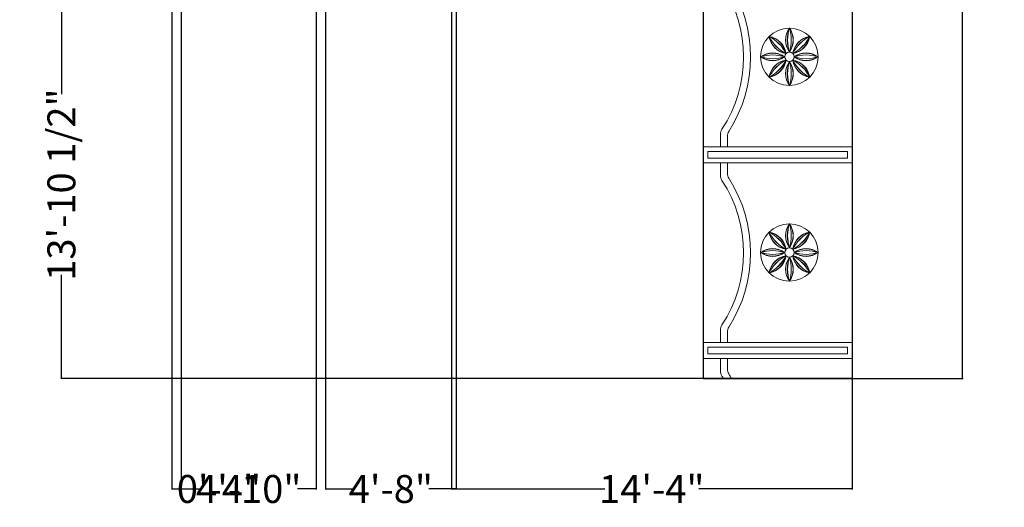
# Model space of a CAD drawing. Units: inches. Extents: x 1146 to 2917, y 889 to 2437.
# Tile 10 of 13: x 2395 to 2817, y 1377 to 1586. Entities that reach past the tile are written whole.
import ezdxf

# ---------------------------------------------------------------- set-up
doc = ezdxf.new("R2010")
doc.units = ezdxf.units.IN
doc.header["$MEASUREMENT"] = 0
for name, color, linetype, lineweight in [('A-ANNO-DIMS', 2, 'Continuous', 18), ('A-ELEV', 7, 'Continuous', 30), ('A-ELEV-ORNM', 8, 'Continuous', 18)]:
    doc.layers.add(name, color=color, linetype=linetype, lineweight=lineweight)
doc.styles.get("Standard").update_dxf_attribs({"font": 'arial.ttf'})
doc.dimstyles.get("Standard").update_dxf_attribs({"dimtxt": 12, "dimasz": 0.18, "dimexe": 0.18, "dimexo": 0.0625, "dimgap": 0.09, "dimtad": 0, "dimtoh": 1, "dimdec": 1, "dimzin": 0, "dimdsep": 46, "dimlunit": 4, "dimtxsty": 'Standard', "dimcen": 0.09, "dimadec": 0, "dimazin": 0, "dimtfac": 1, "dimtdec": 1, "dimtofl": 0, "dimtmove": 0, "dimatfit": 3, "dimfxl": 1, "dimtolj": 1, "dimtzin": 0, "dimarcsym": 0})

# ---------------------------------------------------------------- blocks, each defined once
blk = doc.blocks.new('BOUNDARY-WALL-PIER')
for points in [[(0, 6.94), (64, 6.94), (64, 0), (0, 0)], [(2, 4.94), (62, 4.94), (62, 2), (2, 2)]]:
    blk.add_lwpolyline(points, close=True)
blk = doc.blocks.new('BOUNDARY-WALL-ARCH-CAP')
for p, q in [((0, 71.74), (0, 77.06)), ((3, 72.62), (3, 77.06)), ((0, 0), (0, 5.32)), ((3, 0), (3, 4.44))]:
    blk.add_line(p, q)
for centre, radius, start, end in [((7, 72.62), 4, 180, 212.2708), ((4, 71.74), 4, 180, 213.079), ((-46.98, 38.53), 56.85, 326.921, 33.079), ((-46.98, 38.53), 59.85, 327.7292, 32.2708), ((4, 5.32), 4, 146.921, 180), ((7, 4.44), 4, 147.7292, 180)]:
    blk.add_arc(centre, radius, start, end)
blk = doc.blocks.new('ROSETTE-PLANAR-TRACERY')
for radius in [12.33, 2.02]:
    blk.add_circle((12.33, 12.33), radius)
at = {"extrusion": (-2e-16, 0, -1)}
for centre, radius, start, end in [((-19.47, 19.51), 8.8, 324.1552, 35.8448), ((-4.71, 19.51), 9.21, 145.95, 214.05)]:
    blk.add_arc(centre, radius, start, end, dxfattribs=at)
for centre, radius, start, end in [((19.96, 19.51), 9.21, 145.95, 214.05), ((5.2, 19.51), 8.8, 324.1552, 35.8448), ((2.21, 12.37), 8.8, 9.1552, 80.8448), ((12.65, 22.8), 9.21, 190.95, 259.05), ((12.37, 22.46), 8.8, 279.1552, 350.8448), ((22.8, 12.02), 9.21, 100.95, 169.05), ((5.15, 5.2), 8.8, 54.1552, 125.8448), ((19.51, 4.71), 9.21, 55.95, 124.05), ((5.15, 19.96), 9.21, 235.95, 304.05), ((12.3, 2.21), 8.8, 99.1552, 170.8448), ((1.86, 12.65), 9.21, 280.95, 349.05), ((19.47, 5.15), 8.8, 144.1552, 215.8448), ((4.71, 5.15), 9.21, 325.95, 34.05), ((22.46, 12.3), 8.8, 189.1552, 260.8448), ((12.02, 1.86), 9.21, 10.95, 79.05), ((19.51, 19.47), 8.8, 234.1552, 305.8448)]:
    blk.add_arc(centre, radius, start, end)
at = {"extrusion": (-2e-16, -2e-16, -1)}
for centre, radius, start, end in [((-12.3, 22.46), 8.8, 279.1552, 350.8448), ((-1.86, 12.02), 9.21, 100.95, 169.05)]:
    blk.add_arc(centre, radius, start, end, dxfattribs=at)
at = {"extrusion": (-2e-16, 2e-16, -1)}
for centre, radius, start, end in [((-22.46, 12.37), 8.8, 9.1552, 80.8448), ((-12.02, 22.8), 9.21, 190.95, 259.05)]:
    blk.add_arc(centre, radius, start, end, dxfattribs=at)
at = {"extrusion": (0, -2e-16, -1)}
for centre, radius, start, end in [((-5.15, 4.71), 9.21, 55.95, 124.05), ((-5.15, 19.47), 8.8, 234.1552, 305.8448)]:
    blk.add_arc(centre, radius, start, end, dxfattribs=at)
at = {"extrusion": (0, 2e-16, -1)}
for centre, radius, start, end in [((-19.51, 5.2), 8.8, 54.1552, 125.8448), ((-19.51, 19.96), 9.21, 235.95, 304.05)]:
    blk.add_arc(centre, radius, start, end, dxfattribs=at)
at = {"extrusion": (2e-16, -2e-16, -1)}
for centre, radius, start, end in [((-2.21, 12.3), 8.8, 189.1552, 260.8448), ((-12.65, 1.86), 9.21, 10.95, 79.05)]:
    blk.add_arc(centre, radius, start, end, dxfattribs=at)
at = {"extrusion": (2e-16, 0, -1)}
for centre, radius, start, end in [((-19.96, 5.15), 9.21, 325.95, 34.05), ((-5.2, 5.15), 8.8, 144.1552, 215.8448)]:
    blk.add_arc(centre, radius, start, end, dxfattribs=at)
at = {"extrusion": (2e-16, 2e-16, -1)}
for centre, radius, start, end in [((-12.37, 2.21), 8.8, 99.1552, 170.8448), ((-22.8, 12.65), 9.21, 280.95, 349.05)]:
    blk.add_arc(centre, radius, start, end, dxfattribs=at)
blk = doc.blocks.new('*D121')
at = {"layer": 'A-ANNO-DIMS', "color": 0, "lineweight": -2, "transparency": 16777216}
for p, q in [((2752.26, 2371.39), (2799.78, 2371.39)), ((2799.6, 2371.21), (2799.6, 1936.27)), ((2799.6, 1432.07), (2799.6, 1867.01)), ((2752.26, 1431.89), (2799.78, 1431.89))]:
    blk.add_line(p, q, dxfattribs=at)
at = {"layer": 'A-ANNO-DIMS', "color": 0, "transparency": 16777216}
for points in [[(2799.57, 2371.21), (2799.63, 2371.21), (2799.6, 2371.39)], [(2799.57, 1432.07), (2799.63, 1432.07), (2799.6, 1431.89)]]:
    blk.add_solid(points, dxfattribs=at)
at = {"layer": 'Defpoints', "color": 0, "transparency": 16777216}
for p in [(2752.2, 2371.39), (2799.6, 2371.39), (2752.2, 1431.89)]:
    blk.add_point(p, dxfattribs=at)
at = {"layer": 'A-ANNO-DIMS', "color": 0, "transparency": 16777216, "insert": (2799.6, 1901.64), "char_height": 12, "attachment_point": 5, "rotation": 90}
blk.add_mtext('\\A1;78\'-3 1/2"', dxfattribs=at)
blk = doc.blocks.new('*D128')
at = {"layer": 'A-ANNO-DIMS', "color": 0, "lineweight": -2, "transparency": 16777216}
for p, q in [((2580.2, 1598.33), (2580.2, 1384.31)), ((2752.2, 1431.83), (2752.2, 1384.31)), ((2580.38, 1384.49), (2646.06, 1384.49)), ((2752.02, 1384.49), (2686.34, 1384.49))]:
    blk.add_line(p, q, dxfattribs=at)
at = {"layer": 'A-ANNO-DIMS', "color": 0, "transparency": 16777216}
for points in [[(2580.38, 1384.52), (2580.38, 1384.46), (2580.2, 1384.49)], [(2752.02, 1384.52), (2752.02, 1384.46), (2752.2, 1384.49)]]:
    blk.add_solid(points, dxfattribs=at)
at = {"layer": 'Defpoints', "color": 0, "transparency": 16777216}
for p in [(2580.2, 1598.39), (2752.2, 1431.89), (2752.2, 1384.49)]:
    blk.add_point(p, dxfattribs=at)
at = {"layer": 'A-ANNO-DIMS', "color": 0, "transparency": 16777216, "insert": (2666.2, 1384.49), "char_height": 12, "attachment_point": 5}
blk.add_mtext('\\A1;14\'-4"', dxfattribs=at)
blk = doc.blocks.new('*D129')
at = {"layer": 'A-ANNO-DIMS', "color": 0, "lineweight": -2, "transparency": 16777216}
for p, q in [((2580.14, 1598.39), (2412.62, 1598.39)), ((2412.8, 1598.21), (2412.8, 1553.92)), ((2412.8, 1432.07), (2412.8, 1476.36)), ((2752.14, 1431.89), (2412.62, 1431.89))]:
    blk.add_line(p, q, dxfattribs=at)
at = {"layer": 'A-ANNO-DIMS', "color": 0, "transparency": 16777216}
for points in [[(2412.77, 1598.21), (2412.83, 1598.21), (2412.8, 1598.39)], [(2412.77, 1432.07), (2412.83, 1432.07), (2412.8, 1431.89)]]:
    blk.add_solid(points, dxfattribs=at)
at = {"layer": 'Defpoints', "color": 0, "transparency": 16777216}
for p in [(2580.2, 1598.39), (2412.8, 1431.89), (2752.2, 1431.89)]:
    blk.add_point(p, dxfattribs=at)
at = {"layer": 'A-ANNO-DIMS', "color": 0, "transparency": 16777216, "insert": (2412.8, 1515.14), "char_height": 12, "attachment_point": 5, "rotation": 90}
blk.add_mtext('\\A1;13\'-10 1/2"', dxfattribs=at)
blk = doc.blocks.new('*D133')
at = {"layer": 'A-ANNO-DIMS', "color": 0, "lineweight": -2, "transparency": 16777216}
for p, q in [((2464.2, 1865.33), (2464.2, 1384.31)), ((2522.2, 1865.33), (2522.2, 1384.31)), ((2464.38, 1384.49), (2472.26, 1384.49)), ((2522.02, 1384.49), (2514.14, 1384.49))]:
    blk.add_line(p, q, dxfattribs=at)
at = {"layer": 'A-ANNO-DIMS', "color": 0, "transparency": 16777216}
for points in [[(2464.38, 1384.52), (2464.38, 1384.46), (2464.2, 1384.49)], [(2522.02, 1384.52), (2522.02, 1384.46), (2522.2, 1384.49)]]:
    blk.add_solid(points, dxfattribs=at)
at = {"layer": 'Defpoints', "color": 0, "transparency": 16777216}
for p in [(2464.2, 1865.39), (2522.2, 1865.39), (2522.2, 1384.49)]:
    blk.add_point(p, dxfattribs=at)
at = {"layer": 'A-ANNO-DIMS', "color": 0, "transparency": 16777216, "insert": (2493.2, 1384.49), "char_height": 12, "attachment_point": 5}
blk.add_mtext('\\A1;4\'-10"', dxfattribs=at)
blk = doc.blocks.new('*D134')
at = {"layer": 'A-ANNO-DIMS', "color": 0, "lineweight": -2, "transparency": 16777216}
for p, q in [((2526.2, 1865.33), (2526.2, 1384.31)), ((2582.2, 1865.33), (2582.2, 1384.31)), ((2526.38, 1384.49), (2537.92, 1384.49)), ((2582.02, 1384.49), (2570.48, 1384.49))]:
    blk.add_line(p, q, dxfattribs=at)
at = {"layer": 'A-ANNO-DIMS', "color": 0, "transparency": 16777216}
for points in [[(2526.38, 1384.52), (2526.38, 1384.46), (2526.2, 1384.49)], [(2582.02, 1384.52), (2582.02, 1384.46), (2582.2, 1384.49)]]:
    blk.add_solid(points, dxfattribs=at)
at = {"layer": 'Defpoints', "color": 0, "transparency": 16777216}
for p in [(2526.2, 1865.39), (2582.2, 1865.39), (2582.2, 1384.49)]:
    blk.add_point(p, dxfattribs=at)
at = {"layer": 'A-ANNO-DIMS', "color": 0, "transparency": 16777216, "insert": (2554.2, 1384.49), "char_height": 12, "attachment_point": 5}
blk.add_mtext('\\A1;4\'-8"', dxfattribs=at)
blk = doc.blocks.new('*D135')
at = {"layer": 'A-ANNO-DIMS', "color": 0, "lineweight": -2, "transparency": 16777216}
for p, q in [((2460.2, 1869.33), (2460.2, 1384.31)), ((2464.2, 1865.33), (2464.2, 1384.31)), ((2460.38, 1384.49), (2464.02, 1384.49)), ((2464.2, 1384.49), (2464.38, 1384.49))]:
    blk.add_line(p, q, dxfattribs=at)
at = {"layer": 'A-ANNO-DIMS', "color": 0, "transparency": 16777216}
for points in [[(2460.38, 1384.52), (2460.38, 1384.46), (2460.2, 1384.49)], [(2464.02, 1384.52), (2464.02, 1384.46), (2464.2, 1384.49)]]:
    blk.add_solid(points, dxfattribs=at)
at = {"layer": 'Defpoints', "color": 0, "transparency": 16777216}
for p in [(2460.2, 1869.39), (2464.2, 1865.39), (2464.2, 1384.49)]:
    blk.add_point(p, dxfattribs=at)
at = {"layer": 'A-ANNO-DIMS', "color": 0, "transparency": 16777216, "insert": (2480.42, 1384.49), "char_height": 12, "attachment_point": 5}
blk.add_mtext('\\A1;0\'-4"', dxfattribs=at)

msp = doc.modelspace()

# ---------------------------------------------------------------- linework, layer by layer
at = {"layer": 'A-ELEV'}
for p, q in [((2752.2, 2371.39), (2752.2, 1431.89)), ((2688.2, 2182.39), (2688.2, 1431.89)), ((2688.2, 1431.89), (2752.2, 1431.89))]:
    msp.add_line(p, q, dxfattribs=at)
at = {"layer": 'A-ELEV-ORNM'}
for p, q in [((2695.67, 1435.13), (2695.67, 1440.45)), ((2698.67, 1436.01), (2698.67, 1440.45))]:
    msp.add_line(p, q, dxfattribs=at)
at = {"layer": 'A-ELEV-ORNM', "extrusion": (0.866025, 5.48447e-11, -0.5)}
for centre, radius, start, end in [((1577.18, 1369.76, 2360.14), 8.8, 234.1552, 305.8448), ((1577.18, 1355, 2360.14), 9.21, 55.95, 124.05), ((1493.18, 1369.76, 2360.14), 8.8, 234.1552, 305.8448), ((1493.18, 1355, 2360.14), 9.21, 55.95, 124.05)]:
    msp.add_arc(centre, radius, start, end, dxfattribs=at)
at = {"layer": 'A-ELEV-ORNM', "extrusion": (-0.866025, -5.48447e-11, -0.5)}
for centre, radius, start, end in [((-1577.18, -1369.76, -2360.14), 8.8, 54.1552, 125.8448), ((-1577.18, -1355, -2360.14), 9.21, 235.95, 304.05), ((-1493.18, -1369.76, -2360.14), 8.8, 54.1552, 125.8448), ((-1493.18, -1355, -2360.14), 9.21, 235.95, 304.05)]:
    msp.add_arc(centre, radius, start, end, dxfattribs=at)
at = {"layer": 'A-ELEV-ORNM', "extrusion": (0.866025, 5.48447e-11, 0.5)}
for centre, radius, start, end in [((1577.18, -1370.26, 2360.14), 9.21, 55.95, 124.05), ((1577.18, -1355.49, 2360.14), 8.8, 234.1552, 305.8448), ((1493.18, -1370.26, 2360.14), 9.21, 55.95, 124.05), ((1493.18, -1355.49, 2360.14), 8.8, 234.1552, 305.8448)]:
    msp.add_arc(centre, radius, start, end, dxfattribs=at)
at = {"layer": 'A-ELEV-ORNM', "extrusion": (-0.866025, -5.48447e-11, 0.5)}
for centre, radius, start, end in [((-1577.18, 1370.26, -2360.14), 9.21, 235.95, 304.05), ((-1577.18, 1355.49, -2360.14), 8.8, 54.1552, 125.8448), ((-1493.18, 1370.26, -2360.14), 9.21, 235.95, 304.05), ((-1493.18, 1355.49, -2360.14), 8.8, 54.1552, 125.8448)]:
    msp.add_arc(centre, radius, start, end, dxfattribs=at)
at = {"layer": 'A-ELEV-ORNM', "extrusion": (0.612372, 0.612372, 0.5)}
for centre, radius, start, end in [((-809.71, -1511.47, 2630.3), 8.8, 234.1552, 305.8448), ((-809.71, -1526.23, 2630.3), 9.21, 55.95, 124.05), ((-824.07, -1525.74, 2630.3), 8.8, 54.1552, 125.8448), ((-824.07, -1510.98, 2630.3), 9.21, 235.95, 304.05), ((-869.1, -1481.77, 2578.86), 8.8, 234.1552, 305.8448), ((-869.1, -1496.53, 2578.86), 9.21, 55.95, 124.05), ((-883.46, -1496.04, 2578.86), 8.8, 54.1552, 125.8448), ((-883.46, -1481.28, 2578.86), 9.21, 235.95, 304.05)]:
    msp.add_arc(centre, radius, start, end, dxfattribs=at)
at = {"layer": 'A-ELEV-ORNM', "extrusion": (0.612372, 0.612372, -0.5)}
for centre, radius, start, end in [((-809.71, 1525.74, 2630.3), 8.8, 234.1552, 305.8448), ((-809.71, 1510.98, 2630.3), 9.21, 55.95, 124.05), ((-824.07, 1511.47, 2630.3), 8.8, 54.1552, 125.8448), ((-824.07, 1526.23, 2630.3), 9.21, 235.95, 304.05), ((-869.1, 1496.04, 2578.86), 8.8, 234.1552, 305.8448), ((-869.1, 1481.28, 2578.86), 9.21, 55.95, 124.05), ((-883.46, 1481.77, 2578.86), 8.8, 54.1552, 125.8448), ((-883.46, 1496.53, 2578.86), 9.21, 235.95, 304.05)]:
    msp.add_arc(centre, radius, start, end, dxfattribs=at)
at = {"layer": 'A-ELEV-ORNM', "extrusion": (-0.612372, -0.612372, -0.5)}
for centre, radius, start, end in [((809.71, -1525.74, -2630.3), 8.8, 54.1552, 125.8448), ((809.71, -1510.98, -2630.3), 9.21, 235.95, 304.05), ((824.07, -1511.47, -2630.3), 8.8, 234.1552, 305.8448), ((824.07, -1526.23, -2630.3), 9.21, 55.95, 124.05), ((869.1, -1496.04, -2578.86), 8.8, 54.1552, 125.8448), ((869.1, -1481.28, -2578.86), 9.21, 235.95, 304.05), ((883.46, -1481.77, -2578.86), 8.8, 234.1552, 305.8448), ((883.46, -1496.53, -2578.86), 9.21, 55.95, 124.05)]:
    msp.add_arc(centre, radius, start, end, dxfattribs=at)
at = {"layer": 'A-ELEV-ORNM', "extrusion": (-0.612372, -0.612372, 0.5)}
for centre, radius, start, end in [((809.71, 1511.47, -2630.3), 8.8, 54.1552, 125.8448), ((809.71, 1526.23, -2630.3), 9.21, 235.95, 304.05), ((824.07, 1525.74, -2630.3), 8.8, 234.1552, 305.8448), ((824.07, 1510.98, -2630.3), 9.21, 55.95, 124.05), ((869.1, 1481.77, -2578.86), 8.8, 54.1552, 125.8448), ((869.1, 1496.53, -2578.86), 9.21, 235.95, 304.05), ((883.46, 1496.04, -2578.86), 8.8, 234.1552, 305.8448), ((883.46, 1481.28, -2578.86), 9.21, 55.95, 124.05)]:
    msp.add_arc(centre, radius, start, end, dxfattribs=at)
at = {"layer": 'A-ELEV-ORNM', "extrusion": (0.612372, -0.612372, 0.5)}
for centre, radius, start, end in [((3044.39, -401.31, 707.45), 8.8, 234.1552, 305.8448), ((3044.39, -416.07, 707.45), 9.21, 55.95, 124.05), ((3030.03, -415.58, 707.45), 8.8, 54.1552, 125.8448), ((3030.03, -400.82, 707.45), 9.21, 235.95, 304.05), ((2984.99, -431.01, 758.88), 8.8, 234.1552, 305.8448), ((2984.99, -445.77, 758.88), 9.21, 55.95, 124.05), ((2970.63, -445.28, 758.88), 8.8, 54.1552, 125.8448), ((2970.63, -430.51, 758.88), 9.21, 235.95, 304.05)]:
    msp.add_arc(centre, radius, start, end, dxfattribs=at)
at = {"layer": 'A-ELEV-ORNM', "extrusion": (0.612372, -0.612372, -0.5)}
for centre, radius, start, end in [((3044.39, 415.58, 707.45), 8.8, 234.1552, 305.8448), ((3044.39, 400.82, 707.45), 9.21, 55.95, 124.05), ((3030.03, 401.31, 707.45), 8.8, 54.1552, 125.8448), ((3030.03, 416.07, 707.45), 9.21, 235.95, 304.05), ((2984.99, 445.28, 758.88), 8.8, 234.1552, 305.8448), ((2984.99, 430.51, 758.88), 9.21, 55.95, 124.05), ((2970.63, 431.01, 758.88), 8.8, 54.1552, 125.8448), ((2970.63, 445.77, 758.88), 9.21, 235.95, 304.05)]:
    msp.add_arc(centre, radius, start, end, dxfattribs=at)
at = {"layer": 'A-ELEV-ORNM', "extrusion": (-0.612372, 0.612372, -0.5)}
for centre, radius, start, end in [((-3044.39, -415.58, -707.45), 8.8, 54.1552, 125.8448), ((-3044.39, -400.82, -707.45), 9.21, 235.95, 304.05), ((-3030.03, -401.31, -707.45), 8.8, 234.1552, 305.8448), ((-3030.03, -416.07, -707.45), 9.21, 55.95, 124.05), ((-2984.99, -445.28, -758.88), 8.8, 54.1552, 125.8448), ((-2984.99, -430.51, -758.88), 9.21, 235.95, 304.05), ((-2970.63, -431.01, -758.88), 8.8, 234.1552, 305.8448), ((-2970.63, -445.77, -758.88), 9.21, 55.95, 124.05)]:
    msp.add_arc(centre, radius, start, end, dxfattribs=at)
at = {"layer": 'A-ELEV-ORNM', "extrusion": (-0.612372, 0.612372, 0.5)}
for centre, radius, start, end in [((-3044.39, 401.31, -707.45), 8.8, 54.1552, 125.8448), ((-3044.39, 416.07, -707.45), 9.21, 235.95, 304.05), ((-3030.03, 415.58, -707.45), 8.8, 234.1552, 305.8448), ((-3030.03, 400.82, -707.45), 9.21, 55.95, 124.05), ((-2984.99, 431.01, -758.88), 8.8, 54.1552, 125.8448), ((-2984.99, 445.77, -758.88), 9.21, 235.95, 304.05), ((-2970.63, 445.28, -758.88), 8.8, 234.1552, 305.8448), ((-2970.63, 430.51, -758.88), 9.21, 55.95, 124.05)]:
    msp.add_arc(centre, radius, start, end, dxfattribs=at)
at = {"layer": 'A-ELEV-ORNM', "extrusion": (-5.48444e-11, 0.866025, 0.5)}
for centre, radius, start, end in [((-2718.08, -777.87, 1359.66), 8.8, 234.1552, 305.8448), ((-2718.08, -792.63, 1359.66), 9.21, 55.95, 124.05), ((-2732.44, -777.37, 1359.66), 9.21, 235.95, 304.05), ((-2732.44, -792.14, 1359.66), 8.8, 54.1552, 125.8448), ((-2718.08, -735.87, 1286.92), 8.8, 234.1552, 305.8448), ((-2718.08, -750.63, 1286.92), 9.21, 55.95, 124.05), ((-2732.44, -735.37, 1286.92), 9.21, 235.95, 304.05), ((-2732.44, -750.14, 1286.92), 8.8, 54.1552, 125.8448)]:
    msp.add_arc(centre, radius, start, end, dxfattribs=at)
at = {"layer": 'A-ELEV-ORNM', "extrusion": (5.48444e-11, -0.866025, 0.5)}
for centre, radius, start, end in [((2718.08, 777.87, -1359.66), 8.8, 54.1552, 125.8448), ((2718.08, 792.63, -1359.66), 9.21, 235.95, 304.05), ((2732.44, 777.37, -1359.66), 9.21, 55.95, 124.05), ((2732.44, 792.14, -1359.66), 8.8, 234.1552, 305.8448), ((2718.08, 735.87, -1286.92), 8.8, 54.1552, 125.8448), ((2718.08, 750.63, -1286.92), 9.21, 235.95, 304.05), ((2732.44, 735.37, -1286.92), 9.21, 55.95, 124.05), ((2732.44, 750.14, -1286.92), 8.8, 234.1552, 305.8448)]:
    msp.add_arc(centre, radius, start, end, dxfattribs=at)
at = {"layer": 'A-ELEV-ORNM', "extrusion": (-5.48444e-11, 0.866025, -0.5)}
for centre, radius, start, end in [((-2718.08, 777.37, 1359.66), 9.21, 55.95, 124.05), ((-2718.08, 792.14, 1359.66), 8.8, 234.1552, 305.8448), ((-2732.44, 777.87, 1359.66), 8.8, 54.1552, 125.8448), ((-2732.44, 792.63, 1359.66), 9.21, 235.95, 304.05), ((-2718.08, 735.37, 1286.92), 9.21, 55.95, 124.05), ((-2718.08, 750.14, 1286.92), 8.8, 234.1552, 305.8448), ((-2732.44, 735.87, 1286.92), 8.8, 54.1552, 125.8448), ((-2732.44, 750.63, 1286.92), 9.21, 235.95, 304.05)]:
    msp.add_arc(centre, radius, start, end, dxfattribs=at)
at = {"layer": 'A-ELEV-ORNM', "extrusion": (5.48444e-11, -0.866025, -0.5)}
for centre, radius, start, end in [((2718.08, -777.37, -1359.66), 9.21, 235.95, 304.05), ((2718.08, -792.14, -1359.66), 8.8, 54.1552, 125.8448), ((2732.44, -777.87, -1359.66), 8.8, 234.1552, 305.8448), ((2732.44, -792.63, -1359.66), 9.21, 55.95, 124.05), ((2718.08, -735.37, -1286.92), 9.21, 235.95, 304.05), ((2718.08, -750.14, -1286.92), 8.8, 54.1552, 125.8448), ((2732.44, -735.87, -1286.92), 8.8, 234.1552, 305.8448), ((2732.44, -750.63, -1286.92), 9.21, 55.95, 124.05)]:
    msp.add_arc(centre, radius, start, end, dxfattribs=at)
at = {"layer": 'A-ELEV-ORNM', "extrusion": (-0.866025, -5.48448e-11, 0.5)}
for centre, radius, start, end in [((-1562.82, 1369.76, -2360.14), 8.8, 234.1552, 305.8448), ((-1562.82, 1355, -2360.14), 9.21, 55.95, 124.05), ((-1478.82, 1369.76, -2360.14), 8.8, 234.1552, 305.8448), ((-1478.82, 1355, -2360.14), 9.21, 55.95, 124.05)]:
    msp.add_arc(centre, radius, start, end, dxfattribs=at)
at = {"layer": 'A-ELEV-ORNM', "extrusion": (0.866025, 5.48448e-11, 0.5)}
for centre, radius, start, end in [((1562.82, -1369.76, 2360.14), 8.8, 54.1552, 125.8448), ((1562.82, -1355, 2360.14), 9.21, 235.95, 304.05), ((1478.82, -1369.76, 2360.14), 8.8, 54.1552, 125.8448), ((1478.82, -1355, 2360.14), 9.21, 235.95, 304.05)]:
    msp.add_arc(centre, radius, start, end, dxfattribs=at)
at = {"layer": 'A-ELEV-ORNM', "extrusion": (-0.866025, -5.48448e-11, -0.5)}
for centre, radius, start, end in [((-1562.82, -1370.26, -2360.14), 9.21, 55.95, 124.05), ((-1562.82, -1355.49, -2360.14), 8.8, 234.1552, 305.8448), ((-1478.82, -1370.26, -2360.14), 9.21, 55.95, 124.05), ((-1478.82, -1355.49, -2360.14), 8.8, 234.1552, 305.8448)]:
    msp.add_arc(centre, radius, start, end, dxfattribs=at)
at = {"layer": 'A-ELEV-ORNM', "extrusion": (0.866025, 5.48448e-11, -0.5)}
for centre, radius, start, end in [((1562.82, 1370.26, 2360.14), 9.21, 235.95, 304.05), ((1562.82, 1355.49, 2360.14), 8.8, 54.1552, 125.8448), ((1478.82, 1370.26, 2360.14), 9.21, 235.95, 304.05), ((1478.82, 1355.49, 2360.14), 8.8, 54.1552, 125.8448)]:
    msp.add_arc(centre, radius, start, end, dxfattribs=at)
at = {"layer": 'A-ELEV-ORNM'}
for centre, radius, start, end in [((2699.67, 1435.13), 4, 180, 213.079), ((2648.68, 1401.92), 56.85, 31.8193, 33.079), ((2702.67, 1436.01), 4, 180, 212.2708), ((2648.68, 1401.92), 59.85, 30.0538, 32.2708)]:
    msp.add_arc(centre, radius, start, end, dxfattribs=at)

# ---------------------------------------------------------------- block references
for name, p in [('BOUNDARY-WALL-ARCH-CAP', (2695.67, 1531.39)), ('ROSETTE-PLANAR-TRACERY', (2712.92, 1557.67)), ('BOUNDARY-WALL-PIER', (2688.2, 1524.45)), ('BOUNDARY-WALL-ARCH-CAP', (2695.67, 1447.39)), ('ROSETTE-PLANAR-TRACERY', (2712.92, 1473.67)), ('BOUNDARY-WALL-PIER', (2688.2, 1440.45))]:
    msp.add_blockref(name, p, dxfattribs=at)

# ---------------------------------------------------------------- dimensions: what is measured, and where the dimension line sits
at = {"layer": 'A-ANNO-DIMS'}
for base, p1, p2, picture, middle in [((2799.6, 2371.39), (2752.2, 1431.89), (2752.2, 2371.39), '*D121', (2799.6, 1901.64)), ((2412.8, 1431.89), (2580.2, 1598.39), (2752.2, 1431.89), '*D129', (2412.8, 1515.14))]:
    dim = msp.add_linear_dim(base=base, p1=p1, p2=p2, angle=90, dimstyle='Standard', override={"dimdec": 1, "dimlfac": 1, "dimrnd": 0, "dimzin": 1, "dimdsep": 46, "dimlunit": 4, "dimfrac": 2}, dxfattribs=at)
    dim.commit()
    dim.dimension.update_dxf_attribs({"geometry": picture, "text_midpoint": middle})
for base, p1, p2, picture, middle in [((2464.2, 1384.49), (2460.2, 1869.39), (2464.2, 1865.39), '*D135', (2480.42, 1384.49)), ((2522.2, 1384.49), (2464.2, 1865.39), (2522.2, 1865.39), '*D133', (2493.2, 1384.49)), ((2582.2, 1384.49), (2526.2, 1865.39), (2582.2, 1865.39), '*D134', (2554.2, 1384.49)), ((2752.2, 1384.49), (2580.2, 1598.39), (2752.2, 1431.89), '*D128', (2666.2, 1384.49))]:
    dim = msp.add_linear_dim(base=base, p1=p1, p2=p2, dimstyle='Standard', override={"dimdec": 1, "dimlfac": 1, "dimrnd": 0, "dimzin": 1, "dimdsep": 46, "dimlunit": 4, "dimfrac": 2}, dxfattribs=at)
    dim.commit()
    dim.dimension.update_dxf_attribs({"geometry": picture, "text_midpoint": middle})

doc.saveas('drawing.dxf')
